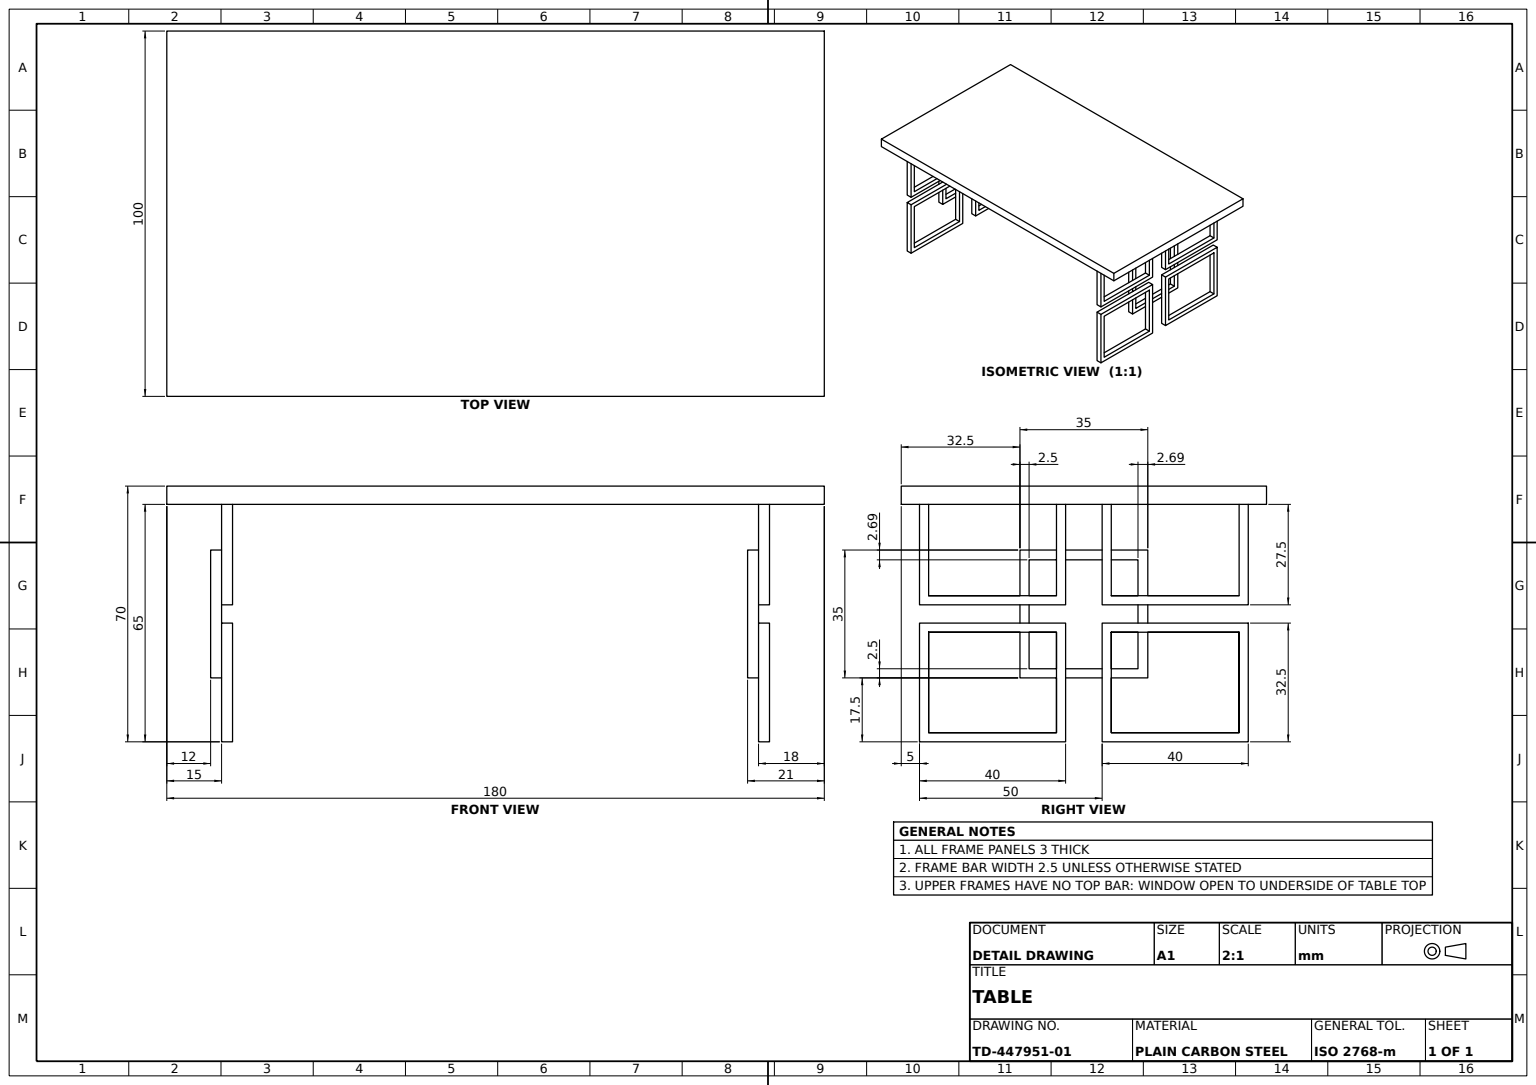
SolidWorks part; units mm, degrees
material "Plain Carbon Steel"
ref_plane "Front Plane" through (0, 0, 0) normal (0, 0, 1) x (1, 0, 0)
ref_plane "Top Plane" through (0, 0, 0) normal (0, 1, 0) x (1, 0, 0)
ref_plane "Right Plane" through (0, 0, 0) normal (1, 0, 0) x (0, 0, -1)
sketch "Front Frame Panel Sketch" plane through (0, 0, 0) normal (0, 0, 1) x (1, 0, 0)
  line L21 (0, 0) -> (40, 0)
  line L22 (0, 0) -> (0, 32.5)
  line L23 (0, 32.5) -> (40, 32.5)
  line L24 (40, 0) -> (40, 32.5)
  dimension "D1" = 40
  dimension "D2" = 32.5
extrude "Front Frame Panel 40x32.5" add sketch "Front Frame Panel Sketch" along normal blind 3
sketch "Front Frame Side Sketch" plane through (0, 0, 3) normal (0, 0, 1) x (1, 0, 0)
  line L0 (20, 0) -> (20, 32.5) construction
  line L1 (0, 0) -> (40, 0) construction
  line L2 (40, 32.5) -> (0, 32.5) construction
  line L5 (40, 0) -> (40, 32.5) construction
  line L7 (50, 32.5) -> (90, 32.5)
  line L8 (50, 32.5) -> (50, 0)
  line L9 (50, 0) -> (90, 0)
  line L10 (90, 32.5) -> (90, 0)
  dimension "D1" = 40
  dimension "D2" = 10
  dimension "D3" = 32.5
extrude "Front Frame Side" add sketch "Front Frame Side Sketch" against normal blind 3 separate body
sketch "Front Frame Outer Sketch" plane through (0, 0, 3) normal (0, 0, 1) x (1, 0, 0)
  line L0 (40, 32.5) -> (0, 32.5) construction
  line L1 (0, 37.5) -> (40, 37.5)
  line L2 (0, 37.5) -> (0, 70)
  line L3 (0, 70) -> (40, 70)
  line L4 (40, 37.5) -> (40, 70)
  line L5 (90, 32.5) -> (50, 32.5) construction
  line L6 (50, 37.5) -> (90, 37.5)
  line L7 (50, 37.5) -> (50, 70)
  line L8 (50, 70) -> (90, 70)
  line L9 (90, 37.5) -> (90, 70)
  dimension "D1" = 40
  dimension "D2" = 32.5
  dimension "D3" = 5
  dimension "D4" = 40
  dimension "D5" = 5
  dimension "D6" = 32.5
  dimension "D7" = 50
extrude "Front Frame Outer" add sketch "Front Frame Outer Sketch" against normal blind 3 separate body
sketch "Frame Window Cut Sketch" plane through (0, 0, 3) normal (0, 0, 1) x (1, 0, 0)
  line L0 (0, 32.5) -> (0, 0) construction
  line L1 (2.5, 30) -> (37.5, 30)
  line L2 (2.5, 30) -> (2.5, 2.5)
  line L3 (2.5, 2.5) -> (37.5, 2.5)
  line L4 (37.5, 30) -> (37.5, 2.5)
  line L5 (40, 32.5) -> (0, 32.5) construction
  line L6 (40, 0) -> (40, 32.5) construction
  line L7 (0, 0) -> (40, 0) construction
  line L8 (50, 0) -> (90, 0) construction
  line L9 (52.5, 30) -> (87.5, 30)
  line L10 (52.5, 30) -> (52.5, 2.5)
  line L11 (52.5, 2.5) -> (87.5, 2.5)
  line L12 (87.5, 30) -> (87.5, 2.5)
  line L13 (90, 0) -> (90, 32.5) construction
  line L14 (90, 32.5) -> (50, 32.5) construction
  line L15 (50, 32.5) -> (50, 0) construction
  line L16 (0, 37.5) -> (40, 37.5) construction
  line L17 (2.5, 67.5) -> (37.5, 67.5)
  line L18 (2.5, 67.5) -> (2.5, 40)
  line L19 (2.5, 40) -> (37.5, 40)
  line L20 (37.5, 67.5) -> (37.5, 40)
  line L21 (0, 70) -> (0, 37.5) construction
  line L22 (40, 37.5) -> (40, 70) construction
  line L23 (40, 70) -> (0, 70) construction
  line L24 (50, 37.5) -> (90, 37.5) construction
  line L25 (52.5, 67.5) -> (87.5, 67.5)
  line L26 (52.5, 67.5) -> (52.5, 40)
  line L27 (52.5, 40) -> (87.5, 40)
  line L28 (87.5, 67.5) -> (87.5, 40)
  line L29 (90, 37.5) -> (90, 70) construction
  line L30 (50, 70) -> (50, 37.5) construction
  line L31 (90, 70) -> (50, 70) construction
  dimension "D1" = 2.5
  dimension "D2" = 2.5
  dimension "D3" = 2.5
  dimension "D4" = 2.5
  dimension "D5" = 2.5
  dimension "D6" = 2.5
  dimension "D7" = 2.5
  dimension "D8" = 2.5
  dimension "D9" = 2.5
  dimension "D10" = 2.5
  dimension "D11" = 2.5
  dimension "D12" = 2.5
  dimension "D13" = 2.5
  dimension "D14" = 2.5
  dimension "D15" = 2.5
  dimension "D16" = 2.5
extrude "Frame Window Cut" cut sketch "Frame Window Cut Sketch" against normal blind 3
sketch "Front Square Frame Sketch" plane through (0, 0, 3) normal (0, 0, 1) x (1, 0, 0)
  line L0 (20, 70) -> (20, 0) construction
  line L3 (70, 70) -> (70, 0) construction
  line L5 (50, 0) -> (90, 0) construction
  line L6 (70, 35) -> (20, 35) construction
  line L7 (2.5, 30) -> (2.5, 2.5) construction
  line L8 (27.5, 17.5) -> (62.5, 17.5)
  line L9 (27.5, 17.5) -> (27.5, 52.5)
  line L10 (27.5, 52.5) -> (62.5, 52.5)
  line L11 (62.5, 17.5) -> (62.5, 52.5)
  line L12 (27.5, 17.5) -> (62.5, 52.5) construction
  line L13 (27.5, 52.5) -> (62.5, 17.5) construction
  line L14 (30.1862, 49.8138) -> (60, 49.8138)
  line L15 (30.1862, 49.8138) -> (30.1862, 20)
  line L16 (30.1862, 20) -> (60, 20)
  line L17 (60, 49.8138) -> (60, 20)
  line L18 (2.5, 2.5) -> (37.5, 2.5) construction
  point P14 (45, 35)
  dimension "D1" = 35
  dimension "D2" = 35
  dimension "D3" = 2.5
  dimension "D4" = 2.5
  dimension "D5" = 17.5
  dimension "D6" = 25
  dimension "D7" = 27.6862
  dimension "D8" = 42.5
  dimension "D9" = 15
  dimension "D10" = 32.5
  dimension "D11" = 47.3138
extrude "Front Square Frame 35x35" add sketch "Front Square Frame Sketch" along normal blind 3
ref_plane "Plane1" through (0, 0, -147) normal (0, 0, 1) x (1, 0, 0)
sketch "Rear Frame A Sketch" plane through (0, 0, -147) normal (0, 0, 1) x (1, 0, 0)
  line L1 (90, 0) -> (50, 0)
  line L2 (90, 0) -> (90, 32.5)
  line L3 (90, 32.5) -> (50, 32.5)
  line L4 (50, 0) -> (50, 32.5)
  line L5 (52.5, 30) -> (87.5, 30)
  line L6 (52.5, 30) -> (52.5, 2.5)
  line L7 (52.5, 2.5) -> (87.5, 2.5)
  line L8 (87.5, 30) -> (87.5, 2.5)
extrude "Rear Frame A" add sketch "Rear Frame A Sketch" along normal blind 3 separate body
ref_plane "Plane2" through (0, 0, -147) normal (0, 0, 1) x (1, 0, 0)
sketch "Rear Frame B Sketch" plane through (0, 0, -147) normal (0, 0, 1) x (1, 0, 0)
  line L1 (0, 32.5) -> (40, 32.5)
  line L2 (0, 32.5) -> (0, 0)
  line L3 (0, 0) -> (40, 0)
  line L4 (40, 32.5) -> (40, 0)
  line L5 (2.5, 30) -> (37.5, 30)
  line L6 (2.5, 30) -> (2.5, 2.5)
  line L7 (2.5, 2.5) -> (37.5, 2.5)
  line L8 (37.5, 30) -> (37.5, 2.5)
extrude "Rear Frame B" add sketch "Rear Frame B Sketch" along normal blind 3 separate body
ref_plane "Plane3" through (0, 0, -147) normal (0, 0, 1) x (1, 0, 0)
sketch "Rear Frame C Sketch" plane through (0, 0, -147) normal (0, 0, 1) x (1, 0, 0)
  line L1 (40, 37.5) -> (0, 37.5)
  line L2 (40, 37.5) -> (40, 70)
  line L3 (40, 70) -> (0, 70)
  line L4 (0, 37.5) -> (0, 70)
  line L5 (2.5, 67.5) -> (37.5, 67.5)
  line L6 (2.5, 67.5) -> (2.5, 40)
  line L7 (2.5, 40) -> (37.5, 40)
  line L8 (37.5, 67.5) -> (37.5, 40)
extrude "Rear Frame C" add sketch "Rear Frame C Sketch" along normal blind 3 separate body
ref_plane "Plane4" through (0, 0, -147) normal (0, 0, 1) x (1, 0, 0)
sketch "Rear Frame D Sketch" plane through (0, 0, -147) normal (0, 0, 1) x (1, 0, 0)
  line L1 (50, 70) -> (90, 70)
  line L2 (50, 70) -> (50, 37.5)
  line L3 (50, 37.5) -> (90, 37.5)
  line L4 (90, 70) -> (90, 37.5)
  line L5 (52.5, 67.5) -> (87.5, 67.5)
  line L6 (52.5, 67.5) -> (52.5, 40)
  line L7 (52.5, 40) -> (87.5, 40)
  line L8 (87.5, 67.5) -> (87.5, 40)
extrude "Rear Frame D" add sketch "Rear Frame D Sketch" along normal blind 3 separate body
sketch "Rear Square Frame Sketch" plane through (0, 0, -144) normal (0, 0, 1) x (1, 0, 0)
  line L1 (27.5, 52.5) -> (62.5, 52.5)
  line L2 (27.5, 52.5) -> (27.5, 17.5)
  line L3 (27.5, 17.5) -> (62.5, 17.5)
  line L4 (62.5, 52.5) -> (62.5, 17.5)
  line L5 (30.1862, 49.8138) -> (60, 49.8138)
  line L6 (30.1862, 49.8138) -> (30.1862, 20)
  line L7 (30.1862, 20) -> (60, 20)
  line L8 (60, 49.8138) -> (60, 20)
extrude "Rear Square Frame" add sketch "Rear Square Frame Sketch" along normal blind 3
sketch "Table Top Sketch" plane through (0, 70, 0) normal (0, 1, 0) x (1, 0, 0)
  line L4 (-5, 0) -> (-5, 162)
  line L5 (-5, 162) -> (95, 162)
  line L6 (95, 162) -> (95, -18)
  line L7 (95, -18) -> (-5, -18)
  line L8 (-5, -18) -> (-5, 0)
  dimension "D1" = 18
  dimension "D2" = 162
  dimension "D3" = 5
  dimension "D4" = 100
extrude "Table Top 162x100x5" add sketch "Table Top Sketch" against normal blind 5
